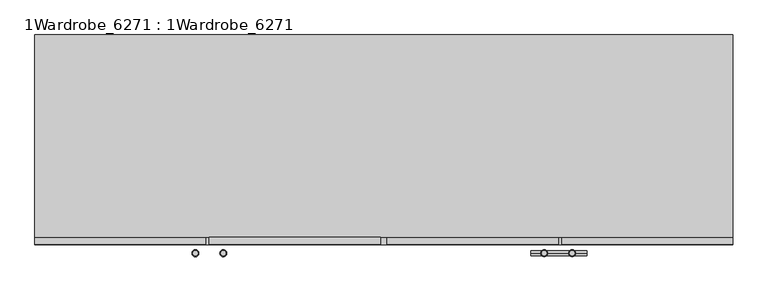
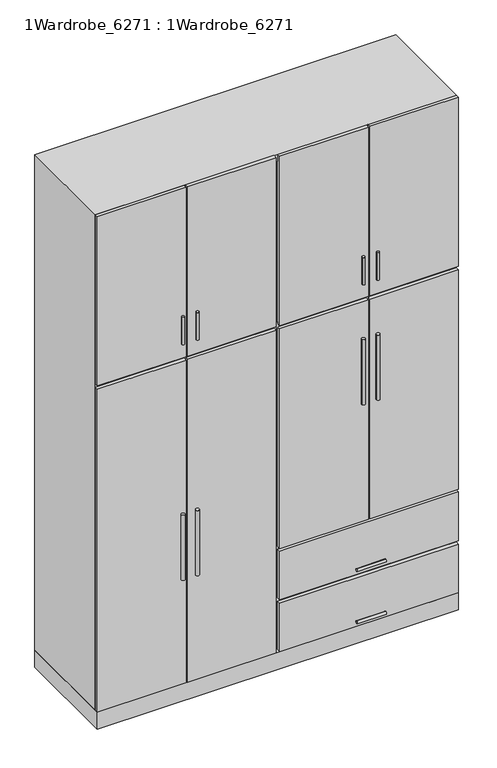
"""IFC4 building model written with IfcOpenShell, lengths in millimetres: furniture geometry, 1Wardrobe_6271 : 1Wardrobe_6271."""

from ifc_helpers import new_model, si_unit, point, frame, frame_2d, origin, origin_with_axes, place, context, project, spatial, polyline, circle_curve, trimmed, segment, composite_curve, outline, extrude, source, transform, mapped, element, save


def furniture_1wardrobe_6271_1wardrobe_6271_4dd35231(model_context):
    return source(origin(), model_context, "Body", "SweptSolid", [
        extrude(outline(polyline([(2000.0, -600.0), (0.0, -600.0), (0.0, 0.0), (2000.0, 0.0), (2000.0, -600.0)])), origin_with_axes(), (0.0, 0.0, 1.0), 100.0),
        extrude(outline(polyline([(490.0, -600.0), (0.0, -600.0), (0.0, -580.0), (490.0, -580.0), (490.0, -600.0)])), frame((0.0, 0.0, 100.0), z_axis=(0.0, 0.0, 1.0), x_axis=(1.0, 0.0, 0.0)), (0.0, 0.0, 1.0), 1890.0),
        extrude(outline(polyline([(990.0, -600.0), (500.0, -600.0), (500.0, -580.0), (990.0, -580.0), (990.0, -600.0)])), frame((0.0, 0.0, 2010.0), z_axis=(0.0, 0.0, 1.0), x_axis=(1.0, 0.0, 0.0)), (0.0, 0.0, 1.0), 990.0),
        extrude(outline(polyline([(2000.0, -600.0), (1010.0, -600.0), (1010.0, -580.0), (2000.0, -580.0), (2000.0, -600.0)])), frame((0.0, 0.0, 100.0), z_axis=(0.0, 0.0, 1.0), x_axis=(1.0, 0.0, 0.0)), (0.0, 0.0, 1.0), 285.0),
        extrude(outline(polyline([(3000.0, 0.0), (100.0, 0.0), (100.0, 40.0), (2960.0, 40.0), (2960.0, 1960.0), (100.0, 1960.0), (100.0, 2000.0), (3000.0, 2000.0), (3000.0, 0.0)])), frame((0.0, -580.0, 0.0), z_axis=(0.0, 1.0, 0.0), x_axis=(0.0, 0.0, 1.0)), (0.0, 0.0, 1.0), 580.0),
        extrude(outline(polyline([(1960.0, -20.0), (40.0, -20.0), (40.0, 0.0), (1960.0, 0.0), (1960.0, -20.0)])), frame((0.0, 0.0, 100.0), z_axis=(0.0, 0.0, 1.0), x_axis=(1.0, 0.0, 0.0)), (0.0, 0.0, 1.0), 2860.0),
        extrude(outline(polyline([(1000.0, -580.0), (960.0, -580.0), (960.0, -20.0), (1000.0, -20.0), (1000.0, -580.0)])), frame((0.0, 0.0, 100.0), z_axis=(0.0, 0.0, 1.0), x_axis=(1.0, 0.0, 0.0)), (0.0, 0.0, 1.0), 2860.0),
        extrude(outline(polyline([(960.0, -580.0), (40.0, -580.0), (40.0, -20.0), (960.0, -20.0), (960.0, -580.0)])), frame((0.0, 0.0, 2500.0), z_axis=(0.0, 0.0, 1.0), x_axis=(1.0, 0.0, 0.0)), (0.0, 0.0, 1.0), 40.0),
        extrude(outline(polyline([(1960.0, -580.0), (950.0, -580.0), (950.0, -20.0), (1960.0, -20.0), (1960.0, -580.0)])), frame((0.0, 0.0, 1980.0), z_axis=(0.0, 0.0, 1.0), x_axis=(1.0, 0.0, 0.0)), (0.0, 0.0, 1.0), 40.0),
        extrude(outline(polyline([(1000.0, -580.0), (40.0, -580.0), (40.0, -20.0), (1000.0, -20.0), (1000.0, -580.0)])), frame((0.0, 0.0, 1980.0), z_axis=(0.0, 0.0, 1.0), x_axis=(1.0, 0.0, 0.0)), (0.0, 0.0, 1.0), 40.0),
        extrude(outline(composite_curve([segment(trimmed(circle_curve(frame_2d((460.0, -625.0)), 10.0), [point((470.0, -625.0))], [point((450.0, -625.0))], False, "CARTESIAN"), True, "CONTINUOUS"), segment(trimmed(circle_curve(frame_2d((460.0, -625.0)), 10.0), [point((450.0, -625.0))], [point((470.0, -625.0))], False, "CARTESIAN"), True, "CONTINUOUS")], self_intersect=False)), frame((0.0, 0.0, 733.2017452), z_axis=(0.0, 0.0, 1.0), x_axis=(1.0, 0.0, 0.0)), (0.0, 0.0, 1.0), 380.0),
        extrude(outline(composite_curve([segment(trimmed(circle_curve(frame_2d((540.0, -625.0)), 10.0), [point((530.0, -625.0))], [point((550.0, -625.0))], False, "CARTESIAN"), True, "CONTINUOUS"), segment(trimmed(circle_curve(frame_2d((540.0, -625.0)), 10.0), [point((550.0, -625.0))], [point((530.0, -625.0))], False, "CARTESIAN"), True, "CONTINUOUS")], self_intersect=False)), frame((0.0, 0.0, 733.2017452), z_axis=(0.0, 0.0, 1.0), x_axis=(1.0, 0.0, 0.0)), (0.0, 0.0, 1.0), 380.0),
        extrude(outline(composite_curve([segment(trimmed(circle_curve(frame_2d((1460.0, -625.0)), 10.0), [point((1470.0, -625.0))], [point((1450.0, -625.0))], False, "CARTESIAN"), True, "CONTINUOUS"), segment(trimmed(circle_curve(frame_2d((1460.0, -625.0)), 10.0), [point((1450.0, -625.0))], [point((1470.0, -625.0))], False, "CARTESIAN"), True, "CONTINUOUS")], self_intersect=False)), frame((0.0, 0.0, 1410.0), z_axis=(0.0, 0.0, 1.0), x_axis=(1.0, 0.0, 0.0)), (0.0, 0.0, 1.0), 380.0),
        extrude(outline(composite_curve([segment(trimmed(circle_curve(frame_2d((1540.0, -625.0)), 10.0), [point((1530.0, -625.0))], [point((1550.0, -625.0))], False, "CARTESIAN"), True, "CONTINUOUS"), segment(trimmed(circle_curve(frame_2d((1540.0, -625.0)), 10.0), [point((1550.0, -625.0))], [point((1530.0, -625.0))], False, "CARTESIAN"), True, "CONTINUOUS")], self_intersect=False)), frame((0.0, 0.0, 1410.0), z_axis=(0.0, 0.0, 1.0), x_axis=(1.0, 0.0, 0.0)), (0.0, 0.0, 1.0), 380.0),
        extrude(outline(polyline([(490.0, -600.0), (0.0, -600.0), (0.0, -580.0), (490.0, -580.0), (490.0, -600.0)])), frame((0.0, 0.0, 2010.0), z_axis=(0.0, 0.0, 1.0), x_axis=(1.0, 0.0, 0.0)), (0.0, 0.0, 1.0), 990.0),
        extrude(outline(polyline([(990.0, -600.0), (500.0, -600.0), (500.0, -580.0), (990.0, -580.0), (990.0, -600.0)])), frame((0.0, 0.0, 100.0), z_axis=(0.0, 0.0, 1.0), x_axis=(1.0, 0.0, 0.0)), (0.0, 0.0, 1.0), 1890.0),
        extrude(outline(polyline([(1500.0, -600.0), (1010.0, -600.0), (1010.0, -580.0), (1500.0, -580.0), (1500.0, -600.0)])), frame((0.0, 0.0, 705.0), z_axis=(0.0, 0.0, 1.0), x_axis=(1.0, 0.0, 0.0)), (0.0, 0.0, 1.0), 1285.0),
        extrude(outline(polyline([(2000.0, -600.0), (1510.0, -600.0), (1510.0, -580.0), (2000.0, -580.0), (2000.0, -600.0)])), frame((0.0, 0.0, 705.0), z_axis=(0.0, 0.0, 1.0), x_axis=(1.0, 0.0, 0.0)), (0.0, 0.0, 1.0), 1285.0),
        extrude(outline(polyline([(1500.0, -600.0), (1010.0, -600.0), (1010.0, -580.0), (1500.0, -580.0), (1500.0, -600.0)])), frame((0.0, 0.0, 2010.0), z_axis=(0.0, 0.0, 1.0), x_axis=(1.0, 0.0, 0.0)), (0.0, 0.0, 1.0), 990.0),
        extrude(outline(composite_curve([segment(trimmed(circle_curve(frame_2d((1540.0564646, -624.9990479)), 7.5), [point((1547.5564646, -624.9990479))], [point((1532.5564646, -624.9990479))], False, "CARTESIAN"), True, "CONTINUOUS"), segment(trimmed(circle_curve(frame_2d((1540.0564646, -624.9990479)), 7.5), [point((1532.5564646, -624.9990479))], [point((1547.5564646, -624.9990479))], False, "CARTESIAN"), True, "CONTINUOUS")], self_intersect=False)), frame((0.0, 0.0, 2110.0), z_axis=(0.0, 0.0, 1.0), x_axis=(1.0, 0.0, 0.0)), (0.0, 0.0, 1.0), 160.0),
        extrude(outline(composite_curve([segment(trimmed(circle_curve(frame_2d((1459.9435354, -624.9990479)), 7.5), [point((1452.4435354, -624.9990479))], [point((1467.4435354, -624.9990479))], False, "CARTESIAN"), True, "CONTINUOUS"), segment(trimmed(circle_curve(frame_2d((1459.9435354, -624.9990479)), 7.5), [point((1467.4435354, -624.9990479))], [point((1452.4435354, -624.9990479))], False, "CARTESIAN"), True, "CONTINUOUS")], self_intersect=False)), frame((0.0, 0.0, 2110.0), z_axis=(0.0, 0.0, 1.0), x_axis=(1.0, 0.0, 0.0)), (0.0, 0.0, 1.0), 160.0),
        extrude(outline(composite_curve([segment(trimmed(circle_curve(frame_2d((459.9435354, -624.9990479)), 7.5), [point((452.4435354, -624.9990479))], [point((467.4435354, -624.9990479))], False, "CARTESIAN"), True, "CONTINUOUS"), segment(trimmed(circle_curve(frame_2d((459.9435354, -624.9990479)), 7.5), [point((467.4435354, -624.9990479))], [point((452.4435354, -624.9990479))], False, "CARTESIAN"), True, "CONTINUOUS")], self_intersect=False)), frame((0.0, 0.0, 2110.0), z_axis=(0.0, 0.0, 1.0), x_axis=(1.0, 0.0, 0.0)), (0.0, 0.0, 1.0), 160.0),
        extrude(outline(composite_curve([segment(trimmed(circle_curve(frame_2d((540.0564646, -624.9990479)), 7.5), [point((547.5564646, -624.9990479))], [point((532.5564646, -624.9990479))], False, "CARTESIAN"), True, "CONTINUOUS"), segment(trimmed(circle_curve(frame_2d((540.0564646, -624.9990479)), 7.5), [point((532.5564646, -624.9990479))], [point((547.5564646, -624.9990479))], False, "CARTESIAN"), True, "CONTINUOUS")], self_intersect=False)), frame((0.0, 0.0, 2110.0), z_axis=(0.0, 0.0, 1.0), x_axis=(1.0, 0.0, 0.0)), (0.0, 0.0, 1.0), 160.0),
        extrude(outline(polyline([(2000.0, -600.0), (1510.0, -600.0), (1510.0, -580.0), (2000.0, -580.0), (2000.0, -600.0)])), frame((0.0, 0.0, 2010.0), z_axis=(0.0, 0.0, 1.0), x_axis=(1.0, 0.0, 0.0)), (0.0, 0.0, 1.0), 990.0),
        extrude(outline(composite_curve([segment(trimmed(circle_curve(frame_2d((-624.9990479, 450.2650104)), 7.5), [point((-624.9990479, 442.7650104))], [point((-624.9990479, 457.7650104))], False, "CARTESIAN"), True, "CONTINUOUS"), segment(trimmed(circle_curve(frame_2d((-624.9990479, 450.2650104)), 7.5), [point((-624.9990479, 457.7650104))], [point((-624.9990479, 442.7650104))], False, "CARTESIAN"), True, "CONTINUOUS")], self_intersect=False)), frame((1421.9497928, 0.0, 0.0), z_axis=(1.0, 0.0, 0.0), x_axis=(0.0, 1.0, 0.0)), (0.0, 0.0, 1.0), 160.0),
        extrude(outline(composite_curve([segment(trimmed(circle_curve(frame_2d((-624.9990479, 145.2650104)), 7.5), [point((-624.9990479, 137.7650104))], [point((-624.9990479, 152.7650104))], False, "CARTESIAN"), True, "CONTINUOUS"), segment(trimmed(circle_curve(frame_2d((-624.9990479, 145.2650104)), 7.5), [point((-624.9990479, 152.7650104))], [point((-624.9990479, 137.7650104))], False, "CARTESIAN"), True, "CONTINUOUS")], self_intersect=False)), frame((1421.9497928, 0.0, 0.0), z_axis=(1.0, 0.0, 0.0), x_axis=(0.0, 1.0, 0.0)), (0.0, 0.0, 1.0), 160.0),
        extrude(outline(polyline([(2000.0, -600.0), (1010.0, -600.0), (1010.0, -580.0), (2000.0, -580.0), (2000.0, -600.0)])), frame((0.0, 0.0, 405.0), z_axis=(0.0, 0.0, 1.0), x_axis=(1.0, 0.0, 0.0)), (0.0, 0.0, 1.0), 285.0),
    ])


if __name__ == "__main__":
    model = new_model("IFC4")
    model_context = context("Model", 3, world=origin())
    ifc_project = project(units=[si_unit("LENGTHUNIT", "METRE", prefix="MILLI")], contexts=[model_context])
    site = spatial("IfcSite", under=ifc_project)
    building = spatial("IfcBuilding", under=site)
    placement = place(None, origin())
    furniture_1wardrobe_6271_1wardrobe_6271_shape = furniture_1wardrobe_6271_1wardrobe_6271_4dd35231(model_context)
    element("IfcFurniture", 1, ObjectType="1Wardrobe_6271 : 1Wardrobe_6271", at=placement, inside=building, context=model_context, shape_type="MappedRepresentation", body=[
        mapped(furniture_1wardrobe_6271_1wardrobe_6271_shape, transform((0.0, 0.0, 0.0), x_axis=(1.0, 0.0, 0.0), y_axis=(0.0, 1.0, 0.0), z_axis=(0.0, 0.0, 1.0))),
    ])
    save(model, "model.ifc")

# Revit data of these elements
# Type "1Wardrobe_6271 : 1Wardrobe_6271"
#   Default Elevation = 0
# Element 1 (IfcFurniture, "1Wardrobe_6271 : 1Wardrobe_6271")
#   Materials on its faces: "Phase - Demo", "Default Wall", "Phase - Exist", "Default"
# Materials
#   "Phase - Demo": class "System", colour RGB 255 0 0, transparency 0.4, Cost = 0
#   "Default Wall": colour RGB 128 128 128, transparency 0, Cost = 0
#   "Phase - Exist": class "System", colour RGB 127 127 127, transparency 0, Cost = 0
#   "Default": colour RGB 127 127 127, transparency 0, Cost = 0
